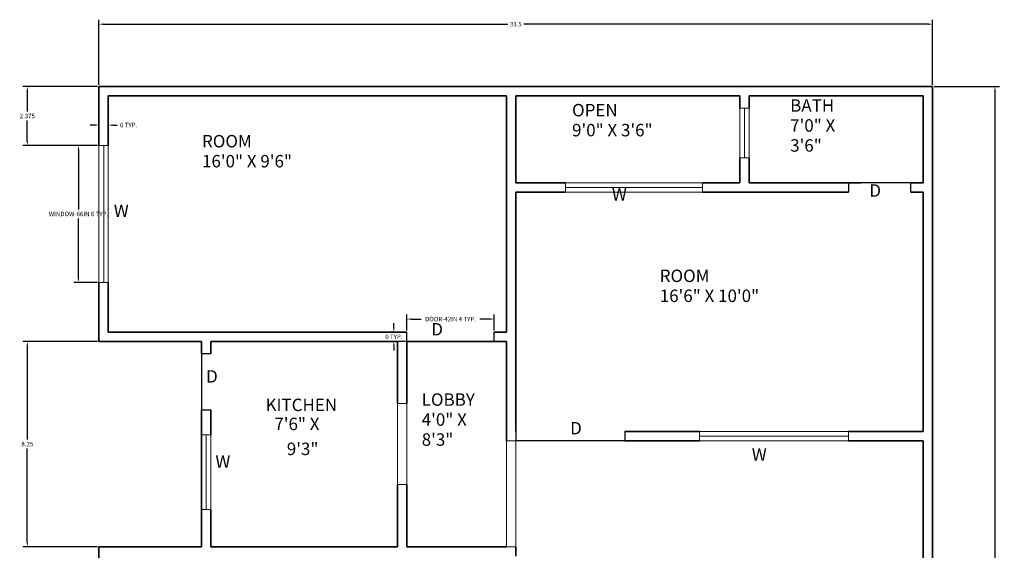
# Model space of a CAD drawing. Units: feet. Extents: x 60.2 to 151.6, y 170.7 to 222.6.
# Tile 3 of 3: x 112 to 151.6, y 201.2 to 222.6. Entities that reach past the tile are written whole.
import ezdxf

# ---------------------------------------------------------------- set-up
doc = ezdxf.new("R2010")
doc.units = ezdxf.units.FT
for name, color, linetype, lineweight in [('A-ANNO-DIMS', 7, 'Continuous', 13), ('A-ANNO-TEXT', 7, 'Continuous', 13), ('A-AREA-IDEN', 7, 'Continuous', 18), ('A-DOOR', 6, 'Continuous', 25), ('A-GLAZ', 240, 'Continuous', 18), ('A-WALL', 175, 'Continuous', 35)]:
    doc.layers.add(name, color=color, linetype=linetype, lineweight=lineweight)
doc.styles.get("Standard").update_dxf_attribs({"font": 'arial.ttf'})
doc.dimstyles.get("Standard").update_dxf_attribs({"dimtxt": 0.18, "dimasz": 0.18, "dimexe": 0.18, "dimexo": 0.0625, "dimgap": 0.09, "dimtad": 0, "dimtih": 1, "dimtoh": 1, "dimdec": 4, "dimzin": 0, "dimdsep": 46, "dimtxsty": 'Standard', "dimcen": 0.09, "dimadec": 0, "dimazin": 0, "dimtfac": 1, "dimtdec": 4, "dimtofl": 0, "dimtmove": 0, "dimatfit": 3, "dimfxl": 1, "dimtolj": 1, "dimtzin": 0, "dimarcsym": 0})

# ---------------------------------------------------------------- blocks, each defined once
blk = doc.blocks.new('DOOR-30IN')
for p, q in [((2.5, 0.375), (0, 0.375)), ((0, 0.375), (0, 0)), ((2.5, 0), (2.5, 0.375))]:
    blk.add_line(p, q)
blk = doc.blocks.new('DOOR-42IN')
for p, q in [((3.5, 0.375), (0, 0.375)), ((0, 0.375), (0, 0)), ((3.5, 0.375), (3.5, 0))]:
    blk.add_line(p, q)
blk = doc.blocks.new('WINDOW-24IN')
for p, q in [((0, 2), (0.375, 2)), ((0, 2), (0, 0)), ((0.188, 2), (0.188, 0)), ((0.375, 2), (0.375, 0)), ((0, 0), (0.375, 0))]:
    blk.add_line(p, q)
blk = doc.blocks.new('WINDOW-66IN')
for p, q in [((0.375, 5.5), (0, 5.5)), ((0, 0), (0, 5.5)), ((0.188, 5.5), (0.188, 0)), ((0.375, 0), (0.375, 5.5)), ((0.375, 0), (0, 0))]:
    blk.add_line(p, q)
blk = doc.blocks.new('WINDOW-36IN')
for p, q in [((0, 0), (0, 3)), ((0, 3), (0.375, 3)), ((0.188, 3), (0.188, 0)), ((0.375, 3), (0.375, 0)), ((0.375, 0), (0, 0))]:
    blk.add_line(p, q)
blk = doc.blocks.new('WINDOW-72IN')
for p, q in [((0, 0.375), (0, 0)), ((6, 0.375), (0, 0.375)), ((0, 0.188), (6, 0.188)), ((6, 0), (0, 0)), ((6, 0), (6, 0.375))]:
    blk.add_line(p, q)
blk = doc.blocks.new('*D18')
at = {"layer": 'A-ANNO-DIMS', "color": 0, "lineweight": -2, "transparency": 16777216}
for p, q in [((127.589, 210.081), (127.589, 210.723)), ((127.769, 210.543), (128.166, 210.543)), ((130.909, 210.543), (130.512, 210.543)), ((131.089, 210.081), (131.089, 210.723))]:
    blk.add_line(p, q, dxfattribs=at)
at = {"layer": 'A-ANNO-DIMS', "color": 0, "transparency": 16777216}
for points in [[(127.769, 210.573), (127.769, 210.513), (127.589, 210.543)], [(130.909, 210.573), (130.909, 210.513), (131.089, 210.543)]]:
    blk.add_solid(points, dxfattribs=at)
at = {"layer": 'Defpoints', "color": 0, "transparency": 16777216}
for p in [(127.589, 210.543), (127.589, 210.018), (131.089, 210.018)]:
    blk.add_point(p, dxfattribs=at)
at = {"layer": 'A-ANNO-DIMS', "color": 0, "transparency": 16777216, "insert": (129.339, 210.543), "char_height": 0.18, "attachment_point": 5}
blk.add_mtext('\\A1;DOOR-42IN 4 TYP.', dxfattribs=at)
blk = doc.blocks.new('*D19')
at = {"layer": 'A-ANNO-DIMS', "color": 0, "lineweight": -2, "transparency": 16777216}
for p, q in [((127.064, 210.198), (127.064, 210.378)), ((127.527, 210.018), (126.884, 210.018)), ((127.527, 209.643), (126.884, 209.643)), ((127.064, 209.463), (127.064, 209.283))]:
    blk.add_line(p, q, dxfattribs=at)
at = {"layer": 'A-ANNO-DIMS', "color": 0, "transparency": 16777216}
for points in [[(127.034, 210.198), (127.094, 210.198), (127.064, 210.018)], [(127.034, 209.463), (127.094, 209.463), (127.064, 209.643)]]:
    blk.add_solid(points, dxfattribs=at)
at = {"layer": 'Defpoints', "color": 0, "transparency": 16777216}
for p in [(127.589, 210.018), (127.064, 209.643), (127.589, 209.643)]:
    blk.add_point(p, dxfattribs=at)
at = {"layer": 'A-ANNO-DIMS', "color": 0, "transparency": 16777216, "insert": (127.064, 209.831), "char_height": 0.18, "attachment_point": 5}
blk.add_mtext('\\A1;0 TYP.', dxfattribs=at)
blk = doc.blocks.new('*D30')
at = {"layer": 'A-ANNO-DIMS', "color": 0, "lineweight": -2, "transparency": 16777216}
for p, q in [((115.152, 217.518), (114.209, 217.518)), ((114.389, 217.338), (114.389, 214.951)), ((114.389, 212.198), (114.389, 214.585)), ((115.152, 212.018), (114.209, 212.018))]:
    blk.add_line(p, q, dxfattribs=at)
at = {"layer": 'A-ANNO-DIMS', "color": 0, "transparency": 16777216}
for points in [[(114.359, 217.338), (114.419, 217.338), (114.389, 217.518)], [(114.359, 212.198), (114.419, 212.198), (114.389, 212.018)]]:
    blk.add_solid(points, dxfattribs=at)
at = {"layer": 'Defpoints', "color": 0, "transparency": 16777216}
for p in [(114.389, 217.518), (115.214, 217.518), (115.214, 212.018)]:
    blk.add_point(p, dxfattribs=at)
at = {"layer": 'A-ANNO-DIMS', "color": 0, "transparency": 16777216, "insert": (114.389, 214.768), "char_height": 0.18, "attachment_point": 5}
blk.add_mtext('\\A1;WINDOW-66IN 6 TYP.', dxfattribs=at)
blk = doc.blocks.new('*D31')
at = {"layer": 'A-ANNO-DIMS', "color": 0, "lineweight": -2, "transparency": 16777216}
for p, q in [((115.214, 217.581), (115.214, 218.523)), ((115.589, 217.581), (115.589, 218.523)), ((115.034, 218.343), (114.854, 218.343)), ((115.769, 218.343), (115.949, 218.343))]:
    blk.add_line(p, q, dxfattribs=at)
at = {"layer": 'A-ANNO-DIMS', "color": 0, "transparency": 16777216}
for points in [[(115.034, 218.373), (115.034, 218.313), (115.214, 218.343)], [(115.769, 218.373), (115.769, 218.313), (115.589, 218.343)]]:
    blk.add_solid(points, dxfattribs=at)
at = {"layer": 'Defpoints', "color": 0, "transparency": 16777216}
for p in [(115.589, 218.343), (115.214, 217.518), (115.589, 217.518)]:
    blk.add_point(p, dxfattribs=at)
at = {"layer": 'A-ANNO-DIMS', "color": 0, "transparency": 16777216, "insert": (116.407, 218.343), "char_height": 0.18, "attachment_point": 5}
blk.add_mtext('\\A1;0 TYP.', dxfattribs=at)
blk = doc.blocks.new('*D45')
at = {"layer": 'A-ANNO-DIMS', "color": 0, "lineweight": -2, "transparency": 16777216}
for p, q in [((148.777, 219.893), (151.399, 219.893)), ((151.219, 219.713), (151.219, 198.388)), ((151.219, 176.698), (151.219, 198.024)), ((148.777, 176.518), (151.399, 176.518))]:
    blk.add_line(p, q, dxfattribs=at)
at = {"layer": 'A-ANNO-DIMS', "color": 0, "transparency": 16777216}
for points in [[(151.189, 219.713), (151.249, 219.713), (151.219, 219.893)], [(151.189, 176.698), (151.249, 176.698), (151.219, 176.518)]]:
    blk.add_solid(points, dxfattribs=at)
at = {"layer": 'Defpoints', "color": 0, "transparency": 16777216}
for p in [(148.714, 219.893), (151.219, 219.893), (148.714, 176.518)]:
    blk.add_point(p, dxfattribs=at)
at = {"layer": 'A-ANNO-DIMS', "color": 0, "transparency": 16777216, "insert": (151.219, 198.206), "char_height": 0.18, "attachment_point": 5}
blk.add_mtext('\\A1;43.375', dxfattribs=at)
blk = doc.blocks.new('*D46')
at = {"layer": 'A-ANNO-DIMS', "color": 0, "lineweight": -2, "transparency": 16777216}
for p, q in [((115.214, 219.956), (115.214, 222.578)), ((115.394, 222.398), (131.64, 222.398)), ((148.534, 222.398), (132.289, 222.398)), ((148.714, 219.956), (148.714, 222.578))]:
    blk.add_line(p, q, dxfattribs=at)
at = {"layer": 'A-ANNO-DIMS', "color": 0, "transparency": 16777216}
for points in [[(115.394, 222.428), (115.394, 222.368), (115.214, 222.398)], [(148.534, 222.428), (148.534, 222.368), (148.714, 222.398)]]:
    blk.add_solid(points, dxfattribs=at)
at = {"layer": 'Defpoints', "color": 0, "transparency": 16777216}
for p in [(148.714, 222.398), (115.214, 219.893), (148.714, 219.893)]:
    blk.add_point(p, dxfattribs=at)
at = {"layer": 'A-ANNO-DIMS', "color": 0, "transparency": 16777216, "insert": (131.964, 222.398), "char_height": 0.18, "attachment_point": 5}
blk.add_mtext('\\A1;33.5', dxfattribs=at)
blk = doc.blocks.new('*D47')
at = {"layer": 'A-ANNO-DIMS', "color": 0, "lineweight": -2, "transparency": 16777216}
for p, q in [((115.152, 209.643), (112.154, 209.643)), ((112.334, 209.463), (112.334, 205.7)), ((112.334, 201.573), (112.334, 205.336)), ((115.152, 201.393), (112.154, 201.393))]:
    blk.add_line(p, q, dxfattribs=at)
at = {"layer": 'A-ANNO-DIMS', "color": 0, "transparency": 16777216}
for points in [[(112.304, 209.463), (112.364, 209.463), (112.334, 209.643)], [(112.304, 201.573), (112.364, 201.573), (112.334, 201.393)]]:
    blk.add_solid(points, dxfattribs=at)
at = {"layer": 'Defpoints', "color": 0, "transparency": 16777216}
for p in [(112.334, 209.643), (115.214, 209.643), (115.214, 201.393)]:
    blk.add_point(p, dxfattribs=at)
at = {"layer": 'A-ANNO-DIMS', "color": 0, "transparency": 16777216, "insert": (112.334, 205.518), "char_height": 0.18, "attachment_point": 5}
blk.add_mtext('\\A1;8.25', dxfattribs=at)
blk = doc.blocks.new('*D48')
at = {"layer": 'A-ANNO-DIMS', "color": 0, "lineweight": -2, "transparency": 16777216}
for p, q in [((115.152, 219.893), (112.154, 219.893)), ((112.334, 219.713), (112.334, 218.888)), ((112.334, 217.698), (112.334, 218.524)), ((115.152, 217.518), (112.154, 217.518))]:
    blk.add_line(p, q, dxfattribs=at)
at = {"layer": 'A-ANNO-DIMS', "color": 0, "transparency": 16777216}
for points in [[(112.304, 219.713), (112.364, 219.713), (112.334, 219.893)], [(112.304, 217.698), (112.364, 217.698), (112.334, 217.518)]]:
    blk.add_solid(points, dxfattribs=at)
at = {"layer": 'Defpoints', "color": 0, "transparency": 16777216}
for p in [(112.334, 219.893), (115.214, 219.893), (115.214, 217.518)]:
    blk.add_point(p, dxfattribs=at)
at = {"layer": 'A-ANNO-DIMS', "color": 0, "transparency": 16777216, "insert": (112.334, 218.706), "char_height": 0.18, "attachment_point": 5}
blk.add_mtext('\\A1;2.375', dxfattribs=at)

msp = doc.modelspace()

# ---------------------------------------------------------------- linework, layer by layer
at = {"layer": 'A-DOOR'}
for p, q in [((145.3392, 216.0182), (145.8392, 216.0182)), ((119.7142, 209.1432), (119.3392, 209.1432)), ((119.3392, 209.1432), (119.3392, 206.8932)), ((119.3392, 206.8932), (119.7142, 206.8932)), ((131.9642, 206.0182), (131.9642, 205.6432)), ((136.3392, 206.0182), (136.3392, 205.6432)), ((136.3392, 205.6432), (131.9642, 205.6432))]:
    msp.add_line(p, q, dxfattribs=at)
at = {"layer": 'A-GLAZ'}
for p, q in [((127.2142, 206.6432), (127.2142, 207.1432)), ((127.2142, 207.1432), (127.5892, 207.1432)), ((127.2142, 207.1432), (127.2142, 203.8932)), ((127.5892, 207.1432), (127.5892, 203.8932)), ((127.5892, 207.1432), (127.5892, 206.6432)), ((131.5892, 201.3932), (131.5892, 205.6432)), ((131.9642, 205.6432), (131.5892, 205.6432)), ((131.9642, 201.3932), (131.9642, 205.6432)), ((141.3392, 205.6432), (139.3392, 205.6432)), ((145.3392, 205.6432), (141.3392, 205.6432)), ((127.2142, 203.8932), (127.5892, 203.8932)), ((131.5892, 201.3932), (131.9642, 201.3932))]:
    msp.add_line(p, q, dxfattribs=at)
at = {"layer": 'A-WALL'}
for p, q in [((115.2142, 219.8932), (145.2142, 219.8932)), ((115.2142, 217.5182), (115.2142, 219.8932)), ((141.3392, 219.8932), (148.3392, 219.8932)), ((148.3392, 219.8932), (148.7142, 219.8932)), ((148.7142, 219.8932), (148.7142, 219.5182)), ((115.5892, 219.5182), (131.5892, 219.5182)), ((115.5892, 219.5182), (131.5892, 219.5182)), ((115.5892, 219.5182), (115.5892, 217.5182)), ((115.5892, 217.5182), (115.5892, 219.5182)), ((131.5892, 219.5182), (131.5892, 210.0182)), ((131.9642, 219.5182), (131.9642, 216.0182)), ((131.9642, 219.5182), (140.9642, 219.5182)), ((131.9642, 219.5182), (140.9642, 219.5182)), ((140.9642, 219.5182), (140.9642, 219.0182)), ((140.9642, 219.5182), (140.9642, 219.0182)), ((141.3392, 219.5182), (141.3392, 219.0182)), ((141.3392, 219.5182), (148.3392, 219.5182)), ((141.3392, 219.5182), (145.2142, 219.5182)), ((148.3392, 219.5182), (148.3392, 216.0182)), ((148.7142, 219.5182), (148.7142, 216.0182)), ((140.9642, 216.0182), (140.9642, 217.0182)), ((140.9642, 217.0182), (140.9642, 216.0182)), ((141.3392, 217.0182), (141.3392, 216.0182)), ((131.9642, 216.0182), (133.9642, 216.0182)), ((133.9642, 216.0182), (131.9642, 216.0182)), ((131.9642, 215.6432), (131.9642, 210.0182)), ((133.9642, 215.6432), (131.9642, 215.6432)), ((140.9642, 216.0182), (139.4642, 216.0182)), ((140.9642, 216.0182), (139.4642, 216.0182)), ((140.9642, 215.6432), (139.4642, 215.6432)), ((140.9642, 215.6432), (141.3392, 215.6432)), ((141.3392, 216.0182), (144.8392, 216.0182)), ((145.3392, 216.0182), (141.3392, 216.0182)), ((145.3392, 215.6432), (141.3392, 215.6432)), ((144.8392, 216.0182), (145.3392, 216.0182)), ((148.3392, 216.0182), (147.8392, 216.0182)), ((148.3392, 216.0182), (147.8392, 216.0182)), ((148.3392, 215.6432), (147.8392, 215.6432)), ((148.3392, 215.6432), (148.3392, 206.0182)), ((148.3392, 215.6432), (148.3392, 206.0182)), ((148.7142, 216.0182), (148.7142, 179.8932)), ((115.2142, 209.6432), (115.2142, 212.0182)), ((115.5892, 210.0182), (115.5892, 212.0182)), ((115.5892, 210.0182), (115.5892, 212.0182)), ((127.5892, 210.0182), (115.5892, 210.0182)), ((131.5892, 210.0182), (131.0892, 210.0182)), ((131.5892, 210.0182), (131.0892, 210.0182)), ((131.9642, 206.0182), (131.9642, 210.0182)), ((115.5892, 209.6432), (115.2142, 209.6432)), ((119.3392, 209.6432), (115.5892, 209.6432)), ((119.3392, 209.6432), (119.3392, 209.1432)), ((127.2142, 209.6432), (119.7142, 209.6432)), ((119.7142, 209.6432), (119.7142, 209.1432)), ((119.7142, 209.6432), (119.7142, 209.1432)), ((127.2142, 209.6432), (119.7142, 209.6432)), ((127.2142, 209.6432), (127.2142, 207.1432)), ((131.5892, 209.6432), (127.5892, 209.6432)), ((127.5892, 209.6432), (127.5892, 207.1432)), ((127.5892, 209.6432), (127.5892, 207.1432)), ((131.5892, 209.6432), (131.0892, 209.6432)), ((131.5892, 205.6432), (131.5892, 209.6432)), ((119.3392, 206.8932), (119.3392, 205.8932)), ((119.3392, 205.8932), (119.3392, 206.8932)), ((119.3392, 206.8932), (119.3392, 201.3932)), ((119.3392, 205.8932), (119.3392, 206.8932)), ((119.7142, 206.8932), (119.7142, 205.8932)), ((137.3392, 206.0182), (136.3392, 206.0182)), ((139.3392, 206.0182), (136.3392, 206.0182)), ((139.3392, 206.0182), (137.3392, 206.0182)), ((148.3392, 206.0182), (145.3392, 206.0182)), ((145.8392, 206.0182), (145.3392, 206.0182)), ((148.3392, 206.0182), (145.8392, 206.0182)), ((139.3392, 205.6432), (136.3392, 205.6432)), ((148.3392, 205.6432), (145.3392, 205.6432)), ((148.3392, 205.6432), (148.3392, 193.2682)), ((127.2142, 203.3932), (127.2142, 203.8932)), ((127.2142, 203.8932), (127.2142, 201.3932)), ((127.5892, 203.8932), (127.5892, 201.3932)), ((127.2142, 201.3932), (127.2142, 203.3932)), ((119.7142, 201.3932), (119.7142, 202.8932)), ((119.7142, 202.8932), (119.7142, 201.3932)), ((115.5892, 201.3932), (115.2142, 201.3932)), ((115.2142, 198.0182), (115.2142, 201.3932)), ((119.3392, 201.3932), (115.5892, 201.3932)), ((119.7142, 201.3932), (127.2142, 201.3932)), ((127.5892, 201.3932), (131.5892, 201.3932)), ((131.9642, 201.3932), (131.9642, 201.0182))]:
    msp.add_line(p, q, dxfattribs=at)

# ---------------------------------------------------------------- block references
at = {"layer": 'A-DOOR'}
msp.add_blockref('DOOR-30IN', (145.3389, 215.643), dxfattribs=at)
at = {"layer": 'A-DOOR', "rotation": 180}
msp.add_blockref('DOOR-42IN', (131.0894, 210.0184), dxfattribs=at)
at = {"layer": 'A-GLAZ'}
for name, p, rotation in [('WINDOW-24IN', (141.3394, 219.0184), 180), ('WINDOW-66IN', (133.964, 216.0184), 270.0000000000014), ('WINDOW-72IN', (145.3394, 206.0184), 180)]:
    msp.add_blockref(name, p, dxfattribs=dict(at, rotation=rotation))
for name, p in [('WINDOW-66IN', (115.214, 212.018)), ('WINDOW-36IN', (119.339, 202.893))]:
    msp.add_blockref(name, p, dxfattribs=at)

# ---------------------------------------------------------------- texts
at = {"layer": 'A-ANNO-DIMS'}
for s, p in [('9\'0" X 3\'6"', (134.2243, 217.8889)), ('7\'0" X ', (142.9889, 218.0759)), ('3\'6"', (142.9889, 217.2727)), ('16\'0" X 9\'6"', (119.3544, 216.6403)), ('16\'6" X 10\'0"', (137.748, 211.2283)), ('7\'6" X ', (122.2616, 206.0776)), ('4\'0" X ', (128.1827, 206.2527)), ('8\'3"', (128.1827, 205.4495)), ('9\'3"', (122.7629, 205.0758))]:
    msp.add_text(s, height=0.5, dxfattribs=at).set_placement(p)
at = {"layer": 'A-ANNO-TEXT'}
for s, p in [('W', (135.8248, 215.3085)), ('D', (146.1731, 215.4619)), ('W', (115.8103, 214.6449)), ('D', (128.5657, 209.8843)), ('D', (119.5181, 207.9888)), ('D', (134.1467, 205.9067)), ('W', (119.8927, 204.5642)), ('W', (141.4471, 204.8462))]:
    msp.add_text(s, height=0.5, dxfattribs=at).set_placement(p)
at = {"layer": 'A-AREA-IDEN'}
for s, p in [('OPEN', (134.2243, 218.6921)), ('BATH', (142.9889, 218.8791)), ('ROOM', (119.3544, 217.4436)), ('ROOM', (137.748, 212.0315)), ('KITCHEN', (121.9077, 206.8436)), ('LOBBY', (128.1827, 207.0559))]:
    msp.add_text(s, height=0.5, dxfattribs=at).set_placement(p)

# ---------------------------------------------------------------- dimensions: what is measured, and where the dimension line sits
at = {"layer": 'A-ANNO-DIMS'}
dim = msp.add_linear_dim(base=(148.7142, 222.3982), p1=(115.2142, 219.8932), p2=(148.7142, 219.8932), dimstyle='Standard', override={"dimdec": 1, "dimlfac": 1, "dimrnd": 0, "dimzin": 0, "dimdsep": 46, "dimlunit": 2}, dxfattribs=at)
dim.commit()
dim.dimension.update_dxf_attribs({"geometry": '*D46', "text_midpoint": (131.9642, 222.3982)})
for base, p1, p2, override, picture, middle in [((112.3342, 219.8932), (115.2142, 217.5182), (115.2142, 219.8932), {"dimdec": 3, "dimlfac": 1, "dimrnd": 0, "dimzin": 0, "dimdsep": 46, "dimlunit": 2}, '*D48', (112.3342, 218.7057)), ((151.2192, 219.8932), (148.7142, 176.5182), (148.7142, 219.8932), {"dimdec": 3, "dimlfac": 1, "dimrnd": 0, "dimzin": 0, "dimdsep": 46, "dimlunit": 2}, '*D45', (151.2192, 198.2057)), ((112.3342, 209.6432), (115.2142, 201.3932), (115.2142, 209.6432), {"dimdec": 2, "dimlfac": 1, "dimrnd": 0, "dimzin": 0, "dimdsep": 46, "dimlunit": 2}, '*D47', (112.3342, 205.5182))]:
    dim = msp.add_linear_dim(base=base, p1=p1, p2=p2, angle=90, dimstyle='Standard', override=override, dxfattribs=at)
    dim.commit()
    dim.dimension.update_dxf_attribs({"geometry": picture, "text_midpoint": middle})
dim = msp.add_linear_dim(base=(115.5892, 218.3432), p1=(115.2142, 217.5182), p2=(115.5892, 217.5182), text='<> TYP.', dimstyle='Standard', override={"dimdec": 0, "dimlfac": 1, "dimrnd": 0, "dimzin": 0, "dimdsep": 46, "dimlunit": 2}, dxfattribs=at)
dim.commit()
dim.dimension.update_dxf_attribs({"geometry": '*D31', "text_midpoint": (116.4073, 218.3432)})
for base, p1, p2, angle, text, picture, middle in [((114.3891535563, 217.5182003807), (115.2141535563, 212.0182003807), (115.2141535563, 217.5182003807), 90, 'WINDOW-66IN <> TYP.', '*D30', (114.3891535563, 214.7682003807)), ((127.5891535563, 210.5432003807), (131.0891535563, 210.0182003807), (127.5891535563, 210.0182003807), 180, 'DOOR-42IN <> TYP.', '*D18', (129.3391535563, 210.5432003807)), ((127.0642, 209.6432), (127.5892, 210.0182), (127.5892, 209.6432), 270, '<> TYP.', '*D19', (127.0642, 209.8307))]:
    dim = msp.add_linear_dim(base=base, p1=p1, p2=p2, angle=angle, text=text, dimstyle='Standard', override={"dimdec": 0, "dimlfac": 1, "dimrnd": 0, "dimzin": 0, "dimdsep": 46, "dimlunit": 2}, dxfattribs=at)
    dim.commit()
    dim.dimension.update_dxf_attribs({"geometry": picture, "text_midpoint": middle})

doc.saveas('drawing.dxf')
